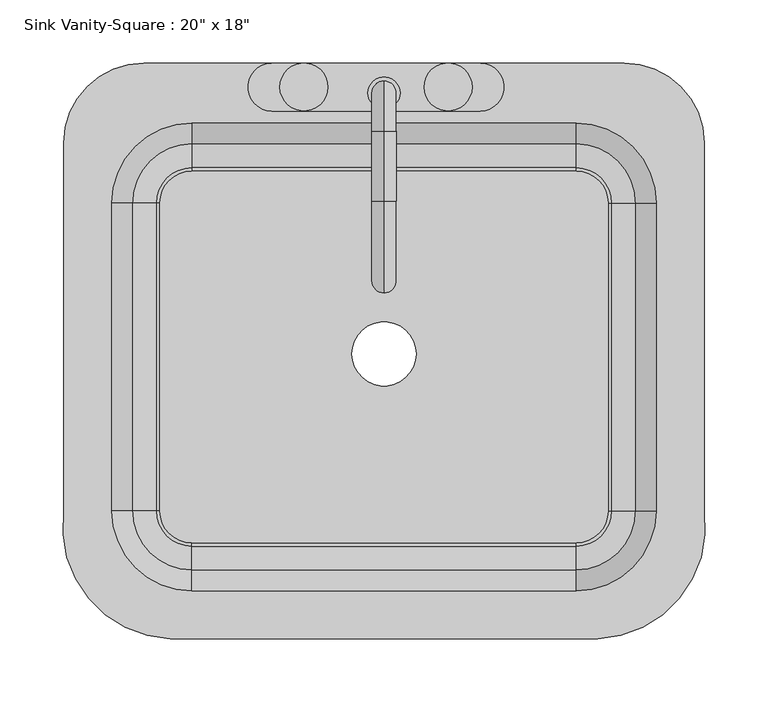
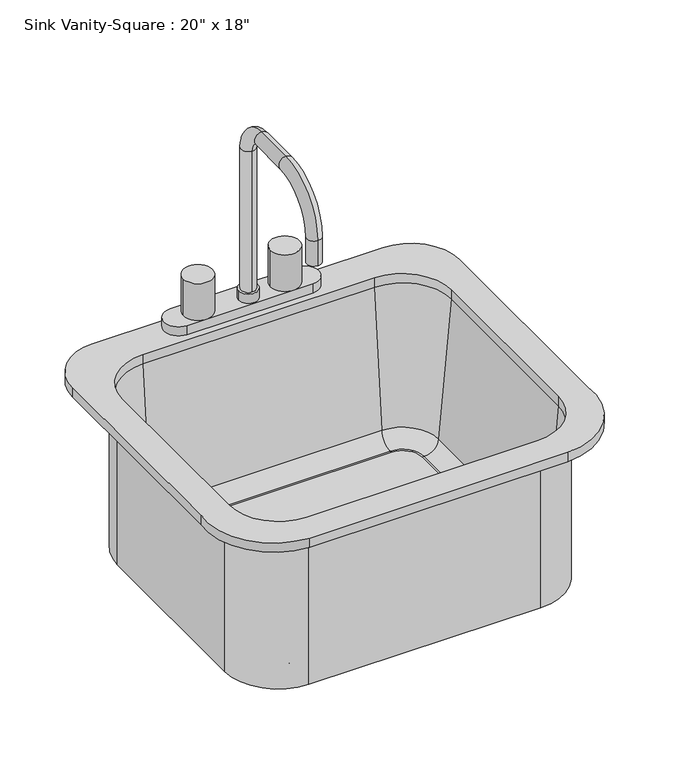
"""IFC4 building model written with IfcOpenShell, lengths in millimetres: flow terminal geometry."""

from ifc_helpers import new_model, si_unit, point, frame, frame_2d, origin, place, context, project, spatial, polyline, circle_curve, ellipse_curve, trimmed, segment, composite_curve, outline, extrude, source, transform, mapped, element, save
from ifc_brep_helpers import plane_surface, cylinder_surface, revolved_surface, advanced_brep


def flow_terminal_8d9ea526(model_context):
    return source(origin(), model_context, "Body", "SolidModel", [
        extrude(outline(composite_curve([segment(trimmed(circle_curve(frame_2d((168.0892406, 69.0204011)), 25.4), [point((168.0892406, 94.4204011))], [point((193.4892406, 69.0204011))], False, "CARTESIAN"), True, "CONTINUOUS"), segment(polyline([(193.4892406, 69.0204011), (193.4892406, -175.4545989)]), True, "CONTINUOUS"), segment(trimmed(circle_curve(frame_2d((168.0892406, -175.4545989)), 25.4), [point((193.4892406, -175.4545989))], [point((168.0892406, -200.8545989))], False, "CARTESIAN"), True, "CONTINUOUS"), segment(polyline([(168.0892406, -200.8545989), (-136.7107594, -200.8545989)]), True, "CONTINUOUS"), segment(trimmed(circle_curve(frame_2d((-136.7107594, -175.4545989)), 25.4), [point((-136.7107594, -200.8545989))], [point((-162.1107594, -175.4545989))], False, "CARTESIAN"), True, "CONTINUOUS"), segment(polyline([(-162.1107594, -175.4545989), (-162.1107594, 69.0204011)]), True, "CONTINUOUS"), segment(trimmed(circle_curve(frame_2d((-136.7107594, 69.0204011)), 25.4), [point((-162.1107594, 69.0204011))], [point((-136.7107594, 94.4204011))], False, "CARTESIAN"), True, "CONTINUOUS"), segment(polyline([(-136.7107594, 94.4204011), (168.0892406, 94.4204011)]), True, "CONTINUOUS")], self_intersect=False), holes=[composite_curve([segment(trimmed(circle_curve(frame_2d((15.6892406, -50.8)), 25.4), [point((-9.7107594, -50.8))], [point((41.0892406, -50.8))], True, "CARTESIAN"), True, "CONTINUOUS"), segment(trimmed(circle_curve(frame_2d((15.6892406, -50.8)), 25.4), [point((41.0892406, -50.8))], [point((-9.7107594, -50.8))], True, "CARTESIAN"), True, "CONTINUOUS")], self_intersect=False)]), frame((0.0, 0.0, 571.5), z_axis=(0.0, 0.0, 1.0), x_axis=(1.0, 0.0, 0.0)), (0.0, 0.0, 1.0), 9.525),
        extrude(outline(composite_curve([segment(trimmed(circle_curve(frame_2d((-47.8107594, 161.0954011)), 19.05), [point((-66.8607594, 161.0954011))], [point((-28.7607594, 161.0954011))], False, "CARTESIAN"), True, "CONTINUOUS"), segment(trimmed(circle_curve(frame_2d((-47.8107594, 161.0954011)), 19.05), [point((-28.7607594, 161.0954011))], [point((-66.8607594, 161.0954011))], False, "CARTESIAN"), True, "CONTINUOUS")], self_intersect=False)), frame((0.0, 0.0, 812.8), z_axis=(0.0, 0.0, 1.0), x_axis=(1.0, 0.0, 0.0)), (0.0, 0.0, 1.0), 50.8),
        extrude(outline(composite_curve([segment(trimmed(circle_curve(frame_2d((66.4892406, 161.0954011)), 19.05), [point((47.4392406, 161.0954011))], [point((85.5392406, 161.0954011))], False, "CARTESIAN"), True, "CONTINUOUS"), segment(trimmed(circle_curve(frame_2d((66.4892406, 161.0954011)), 19.05), [point((85.5392406, 161.0954011))], [point((47.4392406, 161.0954011))], False, "CARTESIAN"), True, "CONTINUOUS")], self_intersect=False)), frame((0.0, 0.0, 812.8), z_axis=(0.0, 0.0, 1.0), x_axis=(1.0, 0.0, 0.0)), (0.0, 0.0, 1.0), 50.8),
        advanced_brep(
        [(91.8892406, 180.1454011, 800.1), (91.8892406, 142.0454011, 800.1), (-73.2107594, 142.0454011, 800.1), (-73.2107594, 180.1454011, 800.1), (15.6892406, 165.8579011, 1020.7625), (15.6892406, 146.8079011, 1020.7625), (15.6892406, 146.8079011, 825.5), (15.6892406, 165.8579011, 825.5), (15.6892406, 126.1704011, 1060.45), (15.6892406, 126.1704011, 1041.4), (15.6892406, 70.6079011, 1060.45), (15.6892406, 70.6079011, 1041.4), (15.6892406, -2.4170989, 987.425), (15.6892406, 16.6329011, 987.425), (15.6892406, -2.4170989, 952.5), (15.6892406, 16.6329011, 952.5), (2.9892406, 156.3329011, 825.5), (28.3892406, 156.3329011, 825.5), (2.9892406, 156.3329011, 812.8), (28.3892406, 156.3329011, 812.8), (91.8892406, 180.1454011, 812.8), (-73.2107594, 180.1454011, 812.8), (-73.2107594, 142.0454011, 812.8), (91.8892406, 142.0454011, 812.8)],
        [
            (0, 1, circle_curve(frame((91.8892406, 161.0954011, 800.1), z_axis=(0.0, 0.0, -1.0), x_axis=(1.0, 0.0, 0.0)), 19.05)),
            (1, 2),
            (2, 3, circle_curve(frame((-73.2107594, 161.0954011, 800.1), z_axis=(0.0, 0.0, -1.0), x_axis=(1.0, 0.0, 0.0)), 19.05)),
            (3, 0),
            (4, 5, circle_curve(frame((15.6892406, 156.3329011, 1020.7625), z_axis=(0.0, 0.0, -1.0), x_axis=(0.0, -1.0, 0.0)), 9.525)),
            (5, 6),
            (6, 7, circle_curve(frame((15.6892406, 156.3329011, 825.5), z_axis=(0.0, 0.0, 1.0), x_axis=(0.0, -1.0, 0.0)), 9.525)),
            (7, 4),
            (5, 4, circle_curve(frame((15.6892406, 156.3329011, 1020.7625), z_axis=(0.0, 0.0, -1.0), x_axis=(0.0, -1.0, 0.0)), 9.525)),
            (7, 6, circle_curve(frame((15.6892406, 156.3329011, 825.5), z_axis=(0.0, 0.0, 1.0), x_axis=(0.0, -1.0, 0.0)), 9.525)),
            (4, 8, circle_curve(frame((15.6892406, 126.1704011, 1020.7625), z_axis=(1.0, 0.0, 0.0), x_axis=(0.0, 1.0, 0.0)), 39.6875)),
            (8, 9, circle_curve(frame((15.6892406, 126.1704011, 1050.925), z_axis=(0.0, 1.0, 0.0), x_axis=(0.0, 0.0, -1.0)), 9.525)),
            (9, 5, circle_curve(frame((15.6892406, 126.1704011, 1020.7625), z_axis=(-1.0, 0.0, 0.0), x_axis=(0.0, 1.0, 0.0)), 20.6375)),
            (9, 8, circle_curve(frame((15.6892406, 126.1704011, 1050.925), z_axis=(0.0, 1.0, 0.0), x_axis=(0.0, 0.0, -1.0)), 9.525)),
            (8, 10),
            (10, 11, circle_curve(frame((15.6892406, 70.6079011, 1050.925), z_axis=(0.0, 1.0, 0.0), x_axis=(0.0, 0.0, -1.0)), 9.525)),
            (11, 9),
            (11, 10, circle_curve(frame((15.6892406, 70.6079011, 1050.925), z_axis=(0.0, 1.0, 0.0), x_axis=(0.0, 0.0, -1.0)), 9.525)),
            (10, 12, circle_curve(frame((15.6892406, 70.6079011, 987.425), z_axis=(1.0, 0.0, 0.0), x_axis=(0.0, 0.0, 1.0)), 73.025)),
            (12, 13, circle_curve(frame((15.6892406, 7.1079011, 987.425), z_axis=(0.0, 0.0, 1.0), x_axis=(0.0, 1.0, 0.0)), 9.525)),
            (13, 11, circle_curve(frame((15.6892406, 70.6079011, 987.425), z_axis=(-1.0, 0.0, 0.0), x_axis=(0.0, 0.0, 1.0)), 53.975)),
            (13, 12, circle_curve(frame((15.6892406, 7.1079011, 987.425), z_axis=(0.0, 0.0, 1.0), x_axis=(0.0, 1.0, 0.0)), 9.525)),
            (14, 15, circle_curve(frame((15.6892406, 7.1079011, 952.5), z_axis=(0.0, 0.0, -1.0), x_axis=(0.0, 1.0, 0.0)), 9.525)),
            (15, 14, circle_curve(frame((15.6892406, 7.1079011, 952.5), z_axis=(0.0, 0.0, -1.0), x_axis=(0.0, 1.0, 0.0)), 9.525)),
            (12, 14),
            (15, 13),
            (16, 17, circle_curve(frame((15.6892406, 156.3329011, 825.5), z_axis=(0.0, 0.0, 1.0), x_axis=(1.0, 0.0, 0.0)), 12.7)),
            (17, 16, circle_curve(frame((15.6892406, 156.3329011, 825.5), z_axis=(0.0, 0.0, 1.0), x_axis=(1.0, 0.0, 0.0)), 12.7)),
            (16, 18),
            (18, 19, circle_curve(frame((15.6892406, 156.3329011, 812.8), z_axis=(0.0, 0.0, 1.0), x_axis=(1.0, 0.0, 0.0)), 12.7)),
            (19, 17),
            (19, 18, circle_curve(frame((15.6892406, 156.3329011, 812.8), z_axis=(0.0, 0.0, 1.0), x_axis=(1.0, 0.0, 0.0)), 12.7)),
            (20, 21),
            (21, 22, circle_curve(frame((-73.2107594, 161.0954011, 812.8), z_axis=(0.0, 0.0, 1.0), x_axis=(1.0, 0.0, 0.0)), 19.05)),
            (22, 23),
            (23, 20, circle_curve(frame((91.8892406, 161.0954011, 812.8), z_axis=(0.0, 0.0, 1.0), x_axis=(1.0, 0.0, 0.0)), 19.05)),
            (20, 0),
            (3, 21),
            (2, 22),
            (1, 23),
        ],
        [
            plane_surface(frame((15.6892406, 146.8079011, 800.1), z_axis=(0.0, 0.0, -1.0), x_axis=(1.0, 0.0, 0.0))),
            cylinder_surface(frame((15.6892406, 156.3329011, 800.1), z_axis=(0.0, 0.0, -1.0), x_axis=(0.0, -1.0, 0.0)), 9.525),
            revolved_surface(trimmed(ellipse_curve(frame((15.6892406, 156.3329011, 1020.7625), z_axis=(0.0, 0.0, -1.0), x_axis=(0.0, -1.0, 0.0)), 9.525, 9.525), [point((15.6892406, 165.8579011, 1020.7625))], [point((15.6892406, 146.8079011, 1020.7625))], True, "CARTESIAN"), (15.6892406, 126.1704011, 1020.7625), (1.0, 0.0, 0.0)),
            revolved_surface(trimmed(ellipse_curve(frame((15.6892406, 156.3329011, 1020.7625), z_axis=(0.0, 0.0, -1.0), x_axis=(0.0, -1.0, 0.0)), 9.525, 9.525), [point((15.6892406, 146.8079011, 1020.7625))], [point((15.6892406, 165.8579011, 1020.7625))], True, "CARTESIAN"), (15.6892406, 126.1704011, 1020.7625), (1.0, 0.0, 0.0)),
            cylinder_surface(frame((15.6892406, 126.1704011, 1050.925), z_axis=(0.0, 1.0, 0.0), x_axis=(0.0, 0.0, -1.0)), 9.525),
            revolved_surface(trimmed(ellipse_curve(frame((15.6892406, 70.6079011, 1050.925), z_axis=(0.0, 1.0, 0.0), x_axis=(0.0, 0.0, -1.0)), 9.525, 9.525), [point((15.6892406, 70.6079011, 1060.45))], [point((15.6892406, 70.6079011, 1041.4))], True, "CARTESIAN"), (15.6892406, 70.6079011, 987.425), (1.0, 0.0, 0.0)),
            revolved_surface(trimmed(ellipse_curve(frame((15.6892406, 70.6079011, 1050.925), z_axis=(0.0, 1.0, 0.0), x_axis=(0.0, 0.0, -1.0)), 9.525, 9.525), [point((15.6892406, 70.6079011, 1041.4))], [point((15.6892406, 70.6079011, 1060.45))], True, "CARTESIAN"), (15.6892406, 70.6079011, 987.425), (1.0, 0.0, 0.0)),
            plane_surface(frame((15.6892406, -2.4170989, 952.5), z_axis=(0.0, 0.0, -1.0), x_axis=(-1.0, 0.0, 0.0))),
            cylinder_surface(frame((15.6892406, 7.1079011, 987.425), z_axis=(0.0, 0.0, 1.0), x_axis=(0.0, 1.0, 0.0)), 9.525),
            plane_surface(frame((28.3892406, 156.3329011, 825.5), z_axis=(0.0, 0.0, 1.0), x_axis=(0.0, 1.0, 0.0))),
            cylinder_surface(frame((15.6892406, 156.3329011, 812.8), z_axis=(0.0, 0.0, 1.0), x_axis=(1.0, 0.0, 0.0)), 12.7),
            plane_surface(frame((-73.2107594, 180.1454011, 812.8), z_axis=(0.0, 0.0, 1.0), x_axis=(-1.0, 0.0, 0.0))),
            plane_surface(frame((91.8892406, 180.1454011, 812.8), z_axis=(0.0, 1.0, 0.0), x_axis=(0.0, 0.0, -1.0))),
            cylinder_surface(frame((-73.2107594, 161.0954011, 800.1), z_axis=(0.0, 0.0, 1.0), x_axis=(1.0, 0.0, 0.0)), 19.05),
            plane_surface(frame((-73.2107594, 142.0454011, 812.8), z_axis=(0.0, -1.0, 0.0), x_axis=(0.0, 0.0, -1.0))),
            cylinder_surface(frame((91.8892406, 161.0954011, 800.1), z_axis=(0.0, 0.0, 1.0), x_axis=(1.0, 0.0, 0.0)), 19.05),
        ],
        [
            (0, [[1, 2, 3, 4]]),
            (1, [[5, 6, 7, 8]]),
            (1, [[9, -8, 10, -6]]),
            (2, [[-5, 11, 12, 13]]),
            (3, [[-9, -13, 14, -11]]),
            (4, [[-12, 15, 16, 17]]),
            (4, [[-14, -17, 18, -15]]),
            (5, [[-16, 19, 20, 21]]),
            (6, [[-18, -21, 22, -19]]),
            (7, [[23, 24]]),
            (8, [[-20, 25, -24, 26]]),
            (8, [[-22, -26, -23, -25]]),
            (9, [[27, 28], [-7, -10]]),
            (10, [[-27, 29, 30, 31]]),
            (10, [[-28, -31, 32, -29]]),
            (11, [[33, 34, 35, 36], [-30, -32]]),
            (12, [[-33, 37, -4, 38]]),
            (13, [[-34, -38, -3, 39]]),
            (14, [[-35, -39, -2, 40]]),
            (15, [[-36, -40, -1, -37]]),
        ],
    ),
        advanced_brep(
        [(-153.9606923, -277.0545989, 800.1), (185.3391735, -277.0545989, 800.1), (269.6892406, -175.4545989, 800.1), (269.6892406, 116.6454011, 800.1), (206.1892406, 180.1454011, 800.1), (-174.8107593, 180.1454011, 800.1), (-238.3107593, 116.6454011, 800.1), (-238.3107593, -175.4545982, 800.1), (168.0892406, 132.5204011, 800.1), (231.5892406, 69.0204011, 800.1), (231.5892406, -175.4545989, 800.1), (168.0892406, -238.9545989, 800.1), (-136.7107594, -238.9545989, 800.1), (-200.2107594, -175.4545989, 800.1), (-200.2107594, 69.0204011, 800.1), (-136.7107594, 132.5204011, 800.1), (-153.9606923, -277.0545989, 787.4), (-238.3107593, -175.4545982, 787.4), (-238.3107593, 116.6454011, 787.4), (-174.8107593, 180.1454011, 787.4), (206.1892406, 180.1454011, 787.4), (269.6892406, 116.6454011, 787.4), (269.6892406, -175.4545989, 787.4), (185.3391735, -277.0545989, 787.4), (237.9392406, 69.0204011, 787.4), (168.0892406, 138.8704011, 787.4), (-136.7107594, 138.8704011, 787.4), (-206.5607594, 69.0204011, 787.4), (-206.5607594, -175.4545989, 787.4), (-136.7107594, -245.3045989, 787.4), (168.0892406, -245.3045989, 787.4), (237.9392406, -175.4545989, 787.4), (168.0892406, 132.5204011, 787.4), (231.5892406, 69.0204011, 787.4), (231.5892406, -175.4545989, 787.4), (168.0892406, -238.9545989, 787.4), (-136.7107594, -238.9545989, 787.4), (-200.2107594, -175.4545989, 787.4), (-200.2107594, 69.0204011, 787.4), (-136.7107594, 132.5204011, 787.4), (237.9392406, 69.0204011, 571.5), (168.0892406, 138.8704011, 571.5), (193.4892406, 69.0204011, 571.5), (168.0892406, 94.4204011, 571.5), (193.4892406, 69.0204011, 581.025), (168.0892406, 94.4204011, 581.025), (196.0776588, 69.0204011, 581.025), (168.0892406, 97.0088193, 581.025), (215.0551678, 69.0204011, 598.4146831), (168.0892406, 115.9863283, 598.4146831), (237.9392406, -175.4545989, 571.5), (193.4892406, -175.4545989, 571.5), (193.4892406, -175.4545989, 581.025), (196.0776588, -175.4545989, 581.025), (215.0551678, -175.4545989, 598.4146831), (168.0892406, -245.3045989, 571.5), (168.0892406, -200.8545989, 571.5), (168.0892406, -200.8545989, 581.025), (168.0892406, -203.4430171, 581.025), (168.0892406, -222.4205261, 598.4146831), (-136.7107594, -245.3045989, 571.5), (-136.7107594, -200.8545989, 571.5), (-136.7107594, -200.8545989, 581.025), (-136.7107594, -203.4430171, 581.025), (-136.7107594, -222.4205261, 598.4146831), (-206.5607594, -175.4545989, 571.5), (-162.1107594, -175.4545989, 571.5), (-162.1107594, -175.4545989, 581.025), (-164.6991776, -175.4545989, 581.025), (-183.6766866, -175.4545989, 598.4146831), (-206.5607594, 69.0204011, 571.5), (-162.1107594, 69.0204011, 571.5), (-162.1107594, 69.0204011, 581.025), (-164.6991776, 69.0204011, 581.025), (-183.6766866, 69.0204011, 598.4146831), (-136.7107594, 138.8704011, 571.5), (-136.7107594, 94.4204011, 571.5), (-136.7107594, 94.4204011, 581.025), (-136.7107594, 97.0088193, 581.025), (-136.7107594, 115.9863283, 598.4146831)],
        [
            (0, 1),
            (1, 2, circle_curve(frame((181.5319557, -188.0793432, 800.1), z_axis=(0.0, 0.0, 1.0), x_axis=(1.0, 0.0, 0.0)), 89.0566732)),
            (2, 3),
            (3, 4, circle_curve(frame((206.1892406, 116.6454011, 800.1), z_axis=(0.0, 0.0, 1.0), x_axis=(1.0, 0.0, 0.0)), 63.5)),
            (4, 5),
            (5, 6, circle_curve(frame((-174.8107593, 116.6454011, 800.1), z_axis=(0.0, 0.0, 1.0), x_axis=(1.0, 0.0, 0.0)), 63.5)),
            (6, 7),
            (7, 0, circle_curve(frame((-150.1534746, -188.0793432, 800.1), z_axis=(0.0, 0.0, 1.0), x_axis=(1.0, 0.0, 0.0)), 89.0566732)),
            (8, 9, circle_curve(frame((168.0892406, 69.0204011, 800.1), z_axis=(0.0, 0.0, -1.0), x_axis=(1.0, 0.0, 0.0)), 63.5)),
            (9, 10),
            (10, 11, circle_curve(frame((168.0892406, -175.4545989, 800.1), z_axis=(0.0, 0.0, -1.0), x_axis=(1.0, 0.0, 0.0)), 63.5)),
            (11, 12),
            (12, 13, circle_curve(frame((-136.7107594, -175.4545989, 800.1), z_axis=(0.0, 0.0, -1.0), x_axis=(1.0, 0.0, 0.0)), 63.5)),
            (13, 14),
            (14, 15, circle_curve(frame((-136.7107594, 69.0204011, 800.1), z_axis=(0.0, 0.0, -1.0), x_axis=(1.0, 0.0, 0.0)), 63.5)),
            (15, 8),
            (16, 17, circle_curve(frame((-150.1534746, -188.0793432, 787.4), z_axis=(0.0, 0.0, -1.0), x_axis=(1.0, 0.0, 0.0)), 89.0566732)),
            (17, 18),
            (18, 19, circle_curve(frame((-174.8107593, 116.6454011, 787.4), z_axis=(0.0, 0.0, -1.0), x_axis=(1.0, 0.0, 0.0)), 63.5)),
            (19, 20),
            (20, 21, circle_curve(frame((206.1892406, 116.6454011, 787.4), z_axis=(0.0, 0.0, -1.0), x_axis=(1.0, 0.0, 0.0)), 63.5)),
            (21, 22),
            (22, 23, circle_curve(frame((181.5319557, -188.0793432, 787.4), z_axis=(0.0, 0.0, -1.0), x_axis=(1.0, 0.0, 0.0)), 89.0566732)),
            (23, 16),
            (24, 25, circle_curve(frame((168.0892406, 69.0204011, 787.4), z_axis=(0.0, 0.0, 1.0), x_axis=(0.0, 1.0, 0.0)), 69.85)),
            (25, 26),
            (26, 27, circle_curve(frame((-136.7107594, 69.0204011, 787.4), z_axis=(0.0, 0.0, 1.0), x_axis=(-1.0, 0.0, 0.0)), 69.85)),
            (27, 28),
            (28, 29, circle_curve(frame((-136.7107594, -175.4545989, 787.4), z_axis=(0.0, 0.0, 1.0), x_axis=(0.0, -1.0, 0.0)), 69.85)),
            (29, 30),
            (30, 31, circle_curve(frame((168.0892406, -175.4545989, 787.4), z_axis=(0.0, 0.0, 1.0), x_axis=(1.0, 0.0, 0.0)), 69.85)),
            (31, 24),
            (0, 16),
            (23, 1),
            (22, 2),
            (21, 3),
            (20, 4),
            (19, 5),
            (18, 6),
            (17, 7),
            (8, 32),
            (32, 33, circle_curve(frame((168.0892406, 69.0204011, 787.4), z_axis=(0.0, 0.0, -1.0), x_axis=(1.0, 0.0, 0.0)), 63.5)),
            (33, 9),
            (33, 34),
            (34, 10),
            (34, 35, circle_curve(frame((168.0892406, -175.4545989, 787.4), z_axis=(0.0, 0.0, -1.0), x_axis=(1.0, 0.0, 0.0)), 63.5)),
            (35, 11),
            (35, 36),
            (36, 12),
            (36, 37, circle_curve(frame((-136.7107594, -175.4545989, 787.4), z_axis=(0.0, 0.0, -1.0), x_axis=(1.0, 0.0, 0.0)), 63.5)),
            (37, 13),
            (37, 38),
            (38, 14),
            (38, 39, circle_curve(frame((-136.7107594, 69.0204011, 787.4), z_axis=(0.0, 0.0, -1.0), x_axis=(1.0, 0.0, 0.0)), 63.5)),
            (39, 15),
            (39, 32),
            (40, 41, circle_curve(frame((168.0892406, 69.0204011, 571.5), z_axis=(0.0, 0.0, 1.0), x_axis=(0.0, 1.0, 0.0)), 69.85)),
            (41, 25),
            (24, 40),
            (40, 42),
            (42, 43, circle_curve(frame((168.0892406, 69.0204011, 571.5), z_axis=(0.0, 0.0, 1.0), x_axis=(0.0, 1.0, 0.0)), 25.4)),
            (43, 41),
            (42, 44),
            (44, 45, circle_curve(frame((168.0892406, 69.0204011, 581.025), z_axis=(0.0, 0.0, 1.0), x_axis=(0.0, 1.0, 0.0)), 25.4)),
            (45, 43),
            (44, 46),
            (46, 47, circle_curve(frame((168.0892406, 69.0204011, 581.025), z_axis=(0.0, 0.0, 1.0), x_axis=(0.0, 1.0, 0.0)), 27.9884182)),
            (47, 45),
            (46, 48, circle_curve(frame((196.0776588, 69.0204011, 600.075), z_axis=(0.0, -1.0, 0.0), x_axis=(1.0, 0.0, 0.0)), 19.05)),
            (48, 49, circle_curve(frame((168.0892406, 69.0204011, 598.4146831), z_axis=(0.0, 0.0, 1.0), x_axis=(0.0, 1.0, 0.0)), 46.9659272)),
            (49, 47, circle_curve(frame((168.0892406, 97.0088193, 600.075), z_axis=(-1.0, 0.0, 0.0), x_axis=(0.0, 1.0, 0.0)), 19.05)),
            (48, 33),
            (32, 49),
            (31, 50),
            (50, 40),
            (50, 51),
            (51, 42),
            (51, 52),
            (52, 44),
            (52, 53),
            (53, 46),
            (53, 54, circle_curve(frame((196.0776588, -175.4545989, 600.075), z_axis=(0.0, -1.0, 0.0), x_axis=(1.0, 0.0, 0.0)), 19.05)),
            (54, 48),
            (54, 34),
            (30, 55),
            (55, 50, circle_curve(frame((168.0892406, -175.4545989, 571.5), z_axis=(0.0, 0.0, 1.0), x_axis=(1.0, 0.0, 0.0)), 69.85)),
            (55, 56),
            (56, 51, circle_curve(frame((168.0892406, -175.4545989, 571.5), z_axis=(0.0, 0.0, 1.0), x_axis=(1.0, 0.0, 0.0)), 25.4)),
            (56, 57),
            (57, 52, circle_curve(frame((168.0892406, -175.4545989, 581.025), z_axis=(0.0, 0.0, 1.0), x_axis=(1.0, 0.0, 0.0)), 25.4)),
            (57, 58),
            (58, 53, circle_curve(frame((168.0892406, -175.4545989, 581.025), z_axis=(0.0, 0.0, 1.0), x_axis=(1.0, 0.0, 0.0)), 27.9884182)),
            (58, 59, circle_curve(frame((168.0892406, -203.4430171, 600.075), z_axis=(-1.0, 0.0, 0.0), x_axis=(0.0, -1.0, 0.0)), 19.05)),
            (59, 54, circle_curve(frame((168.0892406, -175.4545989, 598.4146831), z_axis=(0.0, 0.0, 1.0), x_axis=(1.0, 0.0, 0.0)), 46.9659272)),
            (59, 35),
            (29, 60),
            (60, 55),
            (60, 61),
            (61, 56),
            (61, 62),
            (62, 57),
            (62, 63),
            (63, 58),
            (63, 64, circle_curve(frame((-136.7107594, -203.4430171, 600.075), z_axis=(-1.0, 0.0, 0.0), x_axis=(0.0, -1.0, 0.0)), 19.05)),
            (64, 59),
            (64, 36),
            (28, 65),
            (65, 60, circle_curve(frame((-136.7107594, -175.4545989, 571.5), z_axis=(0.0, 0.0, 1.0), x_axis=(0.0, -1.0, 0.0)), 69.85)),
            (65, 66),
            (66, 61, circle_curve(frame((-136.7107594, -175.4545989, 571.5), z_axis=(0.0, 0.0, 1.0), x_axis=(0.0, -1.0, 0.0)), 25.4)),
            (66, 67),
            (67, 62, circle_curve(frame((-136.7107594, -175.4545989, 581.025), z_axis=(0.0, 0.0, 1.0), x_axis=(0.0, -1.0, 0.0)), 25.4)),
            (67, 68),
            (68, 63, circle_curve(frame((-136.7107594, -175.4545989, 581.025), z_axis=(0.0, 0.0, 1.0), x_axis=(0.0, -1.0, 0.0)), 27.9884182)),
            (68, 69, circle_curve(frame((-164.6991776, -175.4545989, 600.075), z_axis=(0.0, 1.0, 0.0), x_axis=(-1.0, 0.0, 0.0)), 19.05)),
            (69, 64, circle_curve(frame((-136.7107594, -175.4545989, 598.4146831), z_axis=(0.0, 0.0, 1.0), x_axis=(0.0, -1.0, 0.0)), 46.9659272)),
            (69, 37),
            (27, 70),
            (70, 65),
            (70, 71),
            (71, 66),
            (71, 72),
            (72, 67),
            (72, 73),
            (73, 68),
            (73, 74, circle_curve(frame((-164.6991776, 69.0204011, 600.075), z_axis=(0.0, 1.0, 0.0), x_axis=(-1.0, 0.0, 0.0)), 19.05)),
            (74, 69),
            (74, 38),
            (26, 75),
            (75, 70, circle_curve(frame((-136.7107594, 69.0204011, 571.5), z_axis=(0.0, 0.0, 1.0), x_axis=(-1.0, 0.0, 0.0)), 69.85)),
            (75, 76),
            (76, 71, circle_curve(frame((-136.7107594, 69.0204011, 571.5), z_axis=(0.0, 0.0, 1.0), x_axis=(-1.0, 0.0, 0.0)), 25.4)),
            (76, 77),
            (77, 72, circle_curve(frame((-136.7107594, 69.0204011, 581.025), z_axis=(0.0, 0.0, 1.0), x_axis=(-1.0, 0.0, 0.0)), 25.4)),
            (77, 78),
            (78, 73, circle_curve(frame((-136.7107594, 69.0204011, 581.025), z_axis=(0.0, 0.0, 1.0), x_axis=(-1.0, 0.0, 0.0)), 27.9884182)),
            (78, 79, circle_curve(frame((-136.7107594, 97.0088193, 600.075), z_axis=(1.0, 0.0, 0.0), x_axis=(0.0, 1.0, 0.0)), 19.05)),
            (79, 74, circle_curve(frame((-136.7107594, 69.0204011, 598.4146831), z_axis=(0.0, 0.0, 1.0), x_axis=(-1.0, 0.0, 0.0)), 46.9659272)),
            (79, 39),
            (41, 75),
            (43, 76),
            (45, 77),
            (47, 78),
            (49, 79),
        ],
        [
            plane_surface(frame((185.3391735, -277.0545989, 800.1), z_axis=(0.0, 0.0, 1.0), x_axis=(1.0, 0.0, 0.0))),
            plane_surface(frame((185.3391735, -277.0545989, 787.4), z_axis=(0.0, 0.0, -1.0), x_axis=(-1.0, 0.0, 0.0))),
            plane_surface(frame((-153.9606923, -277.0545989, 800.1), z_axis=(0.0, -1.0, 0.0), x_axis=(0.0, 0.0, -1.0))),
            cylinder_surface(frame((181.5319557, -188.0793432, 787.4), z_axis=(0.0, 0.0, 1.0), x_axis=(1.0, 0.0, 0.0)), 89.0566732),
            plane_surface(frame((269.6892406, -175.4545989, 800.1), z_axis=(1.0, 0.0, 0.0), x_axis=(0.0, 0.0, -1.0))),
            cylinder_surface(frame((206.1892406, 116.6454011, 787.4), z_axis=(0.0, 0.0, 1.0), x_axis=(1.0, 0.0, 0.0)), 63.5),
            plane_surface(frame((206.1892406, 180.1454011, 800.1), z_axis=(0.0, 1.0, 0.0), x_axis=(0.0, 0.0, -1.0))),
            cylinder_surface(frame((-174.8107593, 116.6454011, 787.4), z_axis=(0.0, 0.0, 1.0), x_axis=(1.0, 0.0, 0.0)), 63.5),
            plane_surface(frame((-238.3107593, 116.6454011, 800.1), z_axis=(-1.0, 0.0, 0.0), x_axis=(0.0, 0.0, -1.0))),
            cylinder_surface(frame((-150.1534746, -188.0793432, 787.4), z_axis=(0.0, 0.0, 1.0), x_axis=(1.0, 0.0, 0.0)), 89.0566732),
            revolved_surface(polyline([(231.5892406, 69.0204011, 787.4), (231.5892406, 69.0204011, 800.1)]), (168.0892406, 69.0204011, 0.0), (0.0, 0.0, -1.0)),
            plane_surface(frame((231.5892406, 69.0204011, 800.1), z_axis=(-1.0, 0.0, 0.0), x_axis=(0.0, 0.0, -1.0))),
            revolved_surface(polyline([(231.5892406, -175.4545989, 787.4), (231.5892406, -175.4545989, 800.1)]), (168.0892406, -175.4545989, 0.0), (0.0, 0.0, -1.0)),
            plane_surface(frame((168.0892406, -238.9545989, 800.1), z_axis=(0.0, 1.0, 0.0), x_axis=(0.0, 0.0, -1.0))),
            revolved_surface(polyline([(-73.2107594, -175.4545989, 787.4), (-73.2107594, -175.4545989, 800.1)]), (-136.7107594, -175.4545989, 0.0), (0.0, 0.0, -1.0)),
            plane_surface(frame((-200.2107594, -175.4545989, 800.1), z_axis=(1.0, 0.0, 0.0), x_axis=(0.0, 0.0, -1.0))),
            revolved_surface(polyline([(-73.2107594, 69.0204011, 787.4), (-73.2107594, 69.0204011, 800.1)]), (-136.7107594, 69.0204011, 0.0), (0.0, 0.0, -1.0)),
            plane_surface(frame((-136.7107594, 132.5204011, 800.1), z_axis=(0.0, -1.0, 0.0), x_axis=(0.0, 0.0, -1.0))),
            cylinder_surface(frame((168.0892406, 69.0204011, 0.0), z_axis=(0.0, 0.0, -1.0), x_axis=(0.0, 1.0, 0.0)), 69.85),
            plane_surface(frame((168.0892406, 69.0204011, 571.5), z_axis=(0.0, 0.0, -1.0), x_axis=(0.0, 1.0, 0.0))),
            revolved_surface(polyline([(168.0892406, 94.42040109999999, 571.5), (168.0892406, 94.42040109999999, 581.025)]), (168.0892406, 69.0204011, 0.0), (0.0, 0.0, -1.0)),
            plane_surface(frame((168.0892406, 69.0204011, 581.025), z_axis=(0.0, 0.0, 1.0), x_axis=(0.0, 1.0, 0.0))),
            revolved_surface(trimmed(ellipse_curve(frame((168.0892406, 97.0088193, 600.075), z_axis=(1.0, 0.0, 0.0), x_axis=(0.0, 1.0, 0.0)), 19.05, 19.05), [point((168.0892406, 97.0088193, 581.025))], [point((168.0892406, 115.9863283, 598.4146831))], True, "CARTESIAN"), (168.0892406, 69.0204011, 0.0), (0.0, 0.0, -1.0)),
            revolved_surface(polyline([(168.0892406, 115.9863283, 598.4146831), (168.0892406, 132.5204011, 787.4)]), (168.0892406, 69.0204011, 0.0), (0.0, 0.0, -1.0)),
            plane_surface(frame((237.9392406, 69.0204011, 787.4), z_axis=(1.0, 0.0, 0.0), x_axis=(0.0, -1.0, 0.0))),
            plane_surface(frame((237.9392406, 69.0204011, 571.5), z_axis=(0.0, 0.0, -1.0), x_axis=(0.0, -1.0, 0.0))),
            plane_surface(frame((193.4892406, 69.0204011, 571.5), z_axis=(-1.0, 0.0, 0.0), x_axis=(0.0, -1.0, 0.0))),
            plane_surface(frame((193.4892406, 69.0204011, 581.025), z_axis=(0.0, 0.0, 1.0), x_axis=(0.0, -1.0, 0.0))),
            revolved_surface(polyline([(215.1276588, -175.4545989, 600.075), (215.1276588, 69.0204011, 600.075)]), (196.0776588, 69.0204011, 600.075), (0.0, -1.0, 0.0)),
            plane_surface(frame((215.0551678, 69.0204011, 598.4146831), z_axis=(-0.9961946980917442, 0.0, 0.08715574274767397), x_axis=(0.0, -1.0, 0.0))),
            cylinder_surface(frame((168.0892406, -175.4545989, 0.0), z_axis=(0.0, 0.0, -1.0), x_axis=(1.0, 0.0, 0.0)), 69.85),
            plane_surface(frame((168.0892406, -175.4545989, 571.5), z_axis=(0.0, 0.0, -1.0), x_axis=(1.0, 0.0, 0.0))),
            revolved_surface(polyline([(193.48924060000002, -175.4545989, 571.5), (193.48924060000002, -175.4545989, 581.025)]), (168.0892406, -175.4545989, 0.0), (0.0, 0.0, -1.0)),
            plane_surface(frame((168.0892406, -175.4545989, 581.025), z_axis=(0.0, 0.0, 1.0), x_axis=(1.0, 0.0, 0.0))),
            revolved_surface(trimmed(ellipse_curve(frame((196.0776588, -175.4545989, 600.075), z_axis=(0.0, -1.0, 0.0), x_axis=(1.0, 0.0, 0.0)), 19.05, 19.05), [point((196.0776588, -175.4545989, 581.025))], [point((215.0551678, -175.4545989, 598.4146831))], True, "CARTESIAN"), (168.0892406, -175.4545989, 0.0), (0.0, 0.0, -1.0)),
            revolved_surface(polyline([(215.0551678, -175.4545989, 598.4146831), (231.5892406, -175.4545989, 787.4)]), (168.0892406, -175.4545989, 0.0), (0.0, 0.0, -1.0)),
            plane_surface(frame((168.0892406, -245.3045989, 787.4), z_axis=(0.0, -1.0, 0.0), x_axis=(-1.0, 0.0, 0.0))),
            plane_surface(frame((168.0892406, -245.3045989, 571.5), z_axis=(0.0, 0.0, -1.0), x_axis=(-1.0, 0.0, 0.0))),
            plane_surface(frame((168.0892406, -200.8545989, 571.5), z_axis=(0.0, 1.0, 0.0), x_axis=(-1.0, 0.0, 0.0))),
            plane_surface(frame((168.0892406, -200.8545989, 581.025), z_axis=(0.0, 0.0, 1.0), x_axis=(-1.0, 0.0, 0.0))),
            revolved_surface(polyline([(-136.7107594, -222.4930171, 600.075), (168.0892406, -222.4930171, 600.075)]), (168.0892406, -203.4430171, 600.075), (-1.0, 0.0, 0.0)),
            plane_surface(frame((168.0892406, -222.4205261, 598.4146831), z_axis=(0.0, 0.9961946980917442, 0.08715574274767397), x_axis=(-1.0, 0.0, 0.0))),
            cylinder_surface(frame((-136.7107594, -175.4545989, 0.0), z_axis=(0.0, 0.0, -1.0), x_axis=(0.0, -1.0, 0.0)), 69.85),
            plane_surface(frame((-136.7107594, -175.4545989, 571.5), z_axis=(0.0, 0.0, -1.0), x_axis=(0.0, -1.0, 0.0))),
            revolved_surface(polyline([(-136.7107594, -200.8545989, 571.5), (-136.7107594, -200.8545989, 581.025)]), (-136.7107594, -175.4545989, 0.0), (0.0, 0.0, -1.0)),
            plane_surface(frame((-136.7107594, -175.4545989, 581.025), z_axis=(0.0, 0.0, 1.0), x_axis=(0.0, -1.0, 0.0))),
            revolved_surface(trimmed(ellipse_curve(frame((-136.7107594, -203.4430171, 600.075), z_axis=(-1.0, 0.0, 0.0), x_axis=(0.0, -1.0, 0.0)), 19.05, 19.05), [point((-136.7107594, -203.4430171, 581.025))], [point((-136.7107594, -222.4205261, 598.4146831))], True, "CARTESIAN"), (-136.7107594, -175.4545989, 0.0), (0.0, 0.0, -1.0)),
            revolved_surface(polyline([(-136.7107594, -222.4205261, 598.4146831), (-136.7107594, -238.9545989, 787.4)]), (-136.7107594, -175.4545989, 0.0), (0.0, 0.0, -1.0)),
            plane_surface(frame((-206.5607594, -175.4545989, 787.4), z_axis=(-1.0, 0.0, 0.0), x_axis=(0.0, 1.0, 0.0))),
            plane_surface(frame((-206.5607594, -175.4545989, 571.5), z_axis=(0.0, 0.0, -1.0), x_axis=(0.0, 1.0, 0.0))),
            plane_surface(frame((-162.1107594, -175.4545989, 571.5), z_axis=(1.0, 0.0, 0.0), x_axis=(0.0, 1.0, 0.0))),
            plane_surface(frame((-162.1107594, -175.4545989, 581.025), z_axis=(0.0, 0.0, 1.0), x_axis=(0.0, 1.0, 0.0))),
            revolved_surface(polyline([(-183.74917760000002, 69.02040110000002, 600.075), (-183.74917760000002, -175.4545989, 600.075)]), (-164.6991776, -175.4545989, 600.075), (0.0, 1.0, 0.0)),
            plane_surface(frame((-183.6766866, -175.4545989, 598.4146831), z_axis=(0.9961946980917442, 0.0, 0.08715574274767397), x_axis=(0.0, 1.0, 0.0))),
            cylinder_surface(frame((-136.7107594, 69.0204011, 0.0), z_axis=(0.0, 0.0, -1.0), x_axis=(-1.0, 0.0, 0.0)), 69.85),
            plane_surface(frame((-136.7107594, 69.0204011, 571.5), z_axis=(0.0, 0.0, -1.0), x_axis=(-1.0, 0.0, 0.0))),
            revolved_surface(polyline([(-162.1107594, 69.0204011, 571.5), (-162.1107594, 69.0204011, 581.025)]), (-136.7107594, 69.0204011, 0.0), (0.0, 0.0, -1.0)),
            plane_surface(frame((-136.7107594, 69.0204011, 581.025), z_axis=(0.0, 0.0, 1.0), x_axis=(-1.0, 0.0, 0.0))),
            revolved_surface(trimmed(ellipse_curve(frame((-164.6991776, 69.0204011, 600.075), z_axis=(0.0, 1.0, 0.0), x_axis=(-1.0, 0.0, 0.0)), 19.05, 19.05), [point((-164.6991776, 69.0204011, 581.025))], [point((-183.6766866, 69.0204011, 598.4146831))], True, "CARTESIAN"), (-136.7107594, 69.0204011, 0.0), (0.0, 0.0, -1.0)),
            revolved_surface(polyline([(-183.6766866, 69.0204011, 598.4146831), (-200.2107594, 69.0204011, 787.4)]), (-136.7107594, 69.0204011, 0.0), (0.0, 0.0, -1.0)),
            plane_surface(frame((-136.7107594, 138.8704011, 787.4), z_axis=(0.0, 1.0, 0.0), x_axis=(1.0, 0.0, 0.0))),
            plane_surface(frame((-136.7107594, 138.8704011, 571.5), z_axis=(0.0, 0.0, -1.0), x_axis=(1.0, 0.0, 0.0))),
            plane_surface(frame((-136.7107594, 94.4204011, 571.5), z_axis=(0.0, -1.0, 0.0), x_axis=(1.0, 0.0, 0.0))),
            plane_surface(frame((-136.7107594, 94.4204011, 581.025), z_axis=(0.0, 0.0, 1.0), x_axis=(1.0, 0.0, 0.0))),
            revolved_surface(polyline([(168.0892406, 116.0588193, 600.075), (-136.7107594, 116.0588193, 600.075)]), (-136.7107594, 97.0088193, 600.075), (1.0, 0.0, 0.0)),
            plane_surface(frame((-136.7107594, 115.9863283, 598.4146831), z_axis=(0.0, -0.9961946980917442, 0.08715574274767397), x_axis=(1.0, 0.0, 0.0))),
        ],
        [
            (0, [[1, 2, 3, 4, 5, 6, 7, 8], [9, 10, 11, 12, 13, 14, 15, 16]]),
            (1, [[17, 18, 19, 20, 21, 22, 23, 24], [25, 26, 27, 28, 29, 30, 31, 32]]),
            (2, [[-1, 33, -24, 34]]),
            (3, [[-2, -34, -23, 35]]),
            (4, [[-3, -35, -22, 36]]),
            (5, [[-4, -36, -21, 37]]),
            (6, [[-5, -37, -20, 38]]),
            (7, [[-6, -38, -19, 39]]),
            (8, [[-7, -39, -18, 40]]),
            (9, [[-8, -40, -17, -33]]),
            (10, [[-9, 41, 42, 43]]),
            (11, [[-10, -43, 44, 45]]),
            (12, [[-11, -45, 46, 47]]),
            (13, [[-12, -47, 48, 49]]),
            (14, [[-13, -49, 50, 51]]),
            (15, [[-14, -51, 52, 53]]),
            (16, [[-15, -53, 54, 55]]),
            (17, [[-16, -55, 56, -41]]),
            (18, [[57, 58, -25, 59]]),
            (19, [[-57, 60, 61, 62]]),
            (20, [[-61, 63, 64, 65]]),
            (21, [[-64, 66, 67, 68]]),
            (22, [[-67, 69, 70, 71]]),
            (23, [[-70, 72, -42, 73]]),
            (24, [[-59, -32, 74, 75]]),
            (25, [[-60, -75, 76, 77]]),
            (26, [[-63, -77, 78, 79]]),
            (27, [[-66, -79, 80, 81]]),
            (28, [[-69, -81, 82, 83]]),
            (29, [[-72, -83, 84, -44]]),
            (30, [[-74, -31, 85, 86]]),
            (31, [[-76, -86, 87, 88]]),
            (32, [[-78, -88, 89, 90]]),
            (33, [[-80, -90, 91, 92]]),
            (34, [[-82, -92, 93, 94]]),
            (35, [[-84, -94, 95, -46]]),
            (36, [[-85, -30, 96, 97]]),
            (37, [[-87, -97, 98, 99]]),
            (38, [[-89, -99, 100, 101]]),
            (39, [[-91, -101, 102, 103]]),
            (40, [[-93, -103, 104, 105]]),
            (41, [[-95, -105, 106, -48]]),
            (42, [[-96, -29, 107, 108]]),
            (43, [[-98, -108, 109, 110]]),
            (44, [[-100, -110, 111, 112]]),
            (45, [[-102, -112, 113, 114]]),
            (46, [[-104, -114, 115, 116]]),
            (47, [[-106, -116, 117, -50]]),
            (48, [[-107, -28, 118, 119]]),
            (49, [[-109, -119, 120, 121]]),
            (50, [[-111, -121, 122, 123]]),
            (51, [[-113, -123, 124, 125]]),
            (52, [[-115, -125, 126, 127]]),
            (53, [[-117, -127, 128, -52]]),
            (54, [[-118, -27, 129, 130]]),
            (55, [[-120, -130, 131, 132]]),
            (56, [[-122, -132, 133, 134]]),
            (57, [[-124, -134, 135, 136]]),
            (58, [[-126, -136, 137, 138]]),
            (59, [[-128, -138, 139, -54]]),
            (60, [[-58, 140, -129, -26]]),
            (61, [[-62, 141, -131, -140]]),
            (62, [[-65, 142, -133, -141]]),
            (63, [[-68, 143, -135, -142]]),
            (64, [[-71, 144, -137, -143]]),
            (65, [[-73, -56, -139, -144]]),
        ],
    ),
    ])


if __name__ == "__main__":
    model = new_model("IFC4")
    model_context = context("Model", 3, world=origin())
    ifc_project = project(units=[si_unit("LENGTHUNIT", "METRE", prefix="MILLI")], contexts=[model_context])
    site = spatial("IfcSite", under=ifc_project)
    building = spatial("IfcBuilding", under=site)
    placement = place(None, origin())
    flow_terminal_shape = flow_terminal_8d9ea526(model_context)
    element("IfcFlowTerminal", 1, ObjectType="Sink Vanity-Square : 20\" x 18\"", at=placement, inside=building, context=model_context, shape_type="MappedRepresentation", body=[
        mapped(flow_terminal_shape, transform((0.0, 0.0, 0.0), x_axis=(1.0, 0.0, 0.0), y_axis=(0.0, 1.0, 0.0), z_axis=(0.0, 0.0, 1.0))),
    ])
    save(model, "model.ifc")

# Revit data of these elements
# Type "Sink Vanity-Square : 20\" x 18\""
#   Assembly Code = "D2010400"
#   Counter Height = 2' - 7"
#   Depth = 1' - 6"
#   Width = 1' - 8"
#   Basin Material = Porcelain, Linen
#   Faucet Material = Steel, Polished
#   Default Elevation = 0
# Element 1 (IfcFlowTerminal, "Sink Vanity-Square : 20\" x 18\"")
#   Materials on its faces: "Porcelain, Linen", "Steel, Polished"
# Materials
#   "Porcelain, Linen": class "Ceramic", colour RGB 249 239 230, transparency 0, Description = "Porcelain, linen", Cost = 0
#   "Steel, Polished": class "Metal", colour RGB 57 57 57, transparency 0, Description = "Polished steel", Cost = 0
